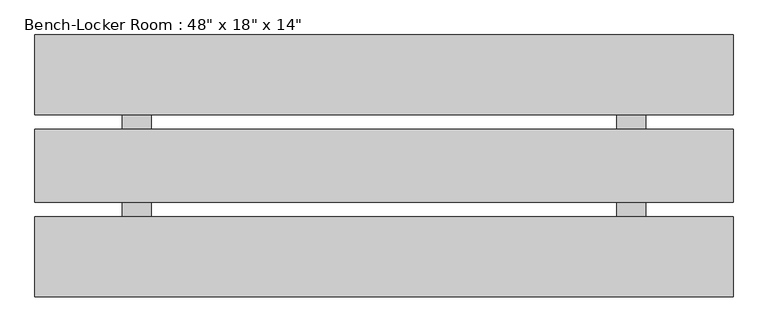
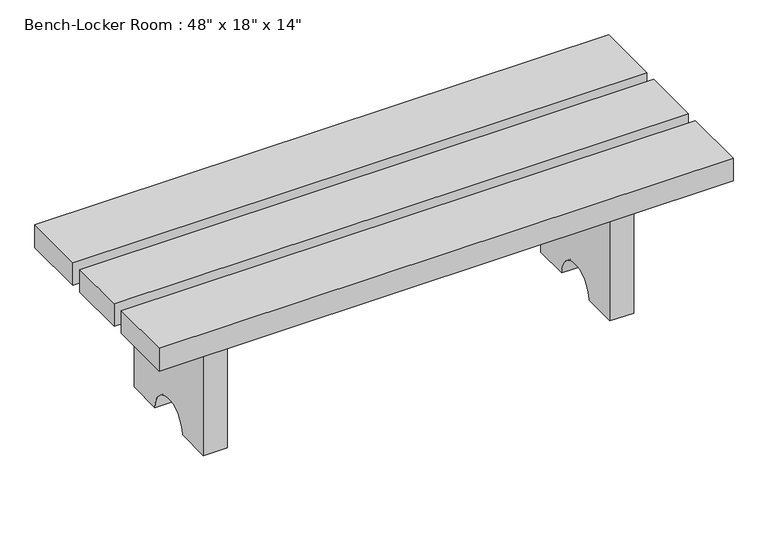
"""IFC4 building model written with IfcOpenShell, lengths in millimetres: furniture geometry."""

from ifc_helpers import new_model, si_unit, point, frame, frame_2d, origin, place, context, project, spatial, polyline, circle_curve, trimmed, segment, composite_curve, outline, extrude, source, transform, mapped, element, save


def furniture_39ce88ff(model_context):
    return source(origin(), model_context, "Body", "SweptSolid", [
        extrude(outline(composite_curve([segment(polyline([(-307.7147541, 0.0), (-307.7147541, 304.8), (-53.7147541, 304.8), (-53.7147541, 0.0), (-129.9147541, 0.0)]), True, "CONTINUOUS"), segment(trimmed(circle_curve(frame_2d((-180.7147541, 0.0)), 50.8), [point((-129.9147541, 0.0))], [point((-231.5147541, 0.0))], True, "CARTESIAN"), True, "CONTINUOUS"), segment(polyline([(-231.5147541, 0.0), (-307.7147541, 0.0)]), True, "CONTINUOUS")], self_intersect=False)), frame((251.0852459, 0.0, 0.0), z_axis=(1.0, 0.0, 0.0), x_axis=(0.0, 1.0, 0.0)), (0.0, 0.0, 1.0), 50.8),
        extrude(outline(composite_curve([segment(polyline([(-53.7147541, 0.0), (-129.9147541, 0.0)]), True, "CONTINUOUS"), segment(trimmed(circle_curve(frame_2d((-180.7147541, 0.0)), 50.8), [point((-129.9147541, 0.0))], [point((-231.5147541, 0.0))], True, "CARTESIAN"), True, "CONTINUOUS"), segment(polyline([(-231.5147541, 0.0), (-307.7147541, 0.0), (-307.7147541, 304.8), (-53.7147541, 304.8), (-53.7147541, 0.0)]), True, "CONTINUOUS")], self_intersect=False)), frame((-612.5147541, 0.0, 0.0), z_axis=(1.0, 0.0, 0.0), x_axis=(0.0, 1.0, 0.0)), (0.0, 0.0, 1.0), 50.8),
        extrude(outline(polyline([(454.2852459, 47.8852459), (454.2852459, -91.8147541), (-764.9147541, -91.8147541), (-764.9147541, 47.8852459), (454.2852459, 47.8852459)])), frame((0.0, 0.0, 304.8), z_axis=(0.0, 0.0, 1.0), x_axis=(1.0, 0.0, 0.0)), (0.0, 0.0, 1.0), 50.8),
        extrude(outline(polyline([(454.2852459, -409.3147541), (-764.9147541, -409.3147541), (-764.9147541, -269.6147541), (454.2852459, -269.6147541), (454.2852459, -409.3147541)])), frame((0.0, 0.0, 304.8), z_axis=(0.0, 0.0, 1.0), x_axis=(1.0, 0.0, 0.0)), (0.0, 0.0, 1.0), 50.8),
        extrude(outline(polyline([(454.2852459, -117.2147541), (454.2852459, -244.2147541), (-764.9147541, -244.2147541), (-764.9147541, -117.2147541), (454.2852459, -117.2147541)])), frame((0.0, 0.0, 304.8), z_axis=(0.0, 0.0, 1.0), x_axis=(1.0, 0.0, 0.0)), (0.0, 0.0, 1.0), 50.8),
    ])


if __name__ == "__main__":
    model = new_model("IFC4")
    model_context = context("Model", 3, world=origin())
    ifc_project = project(units=[si_unit("LENGTHUNIT", "METRE", prefix="MILLI")], contexts=[model_context])
    site = spatial("IfcSite", under=ifc_project)
    building = spatial("IfcBuilding", under=site)
    placement = place(None, origin())
    furniture_shape = furniture_39ce88ff(model_context)
    element("IfcFurniture", 1, ObjectType="Bench-Locker Room : 48\" x 18\" x 14\"", at=placement, inside=building, context=model_context, shape_type="MappedRepresentation", body=[
        mapped(furniture_shape, transform((0.0, 0.0, 0.0), x_axis=(1.0, 0.0, 0.0), y_axis=(0.0, 1.0, 0.0), z_axis=(0.0, 0.0, 1.0))),
    ])
    save(model, "model.ifc")

# Revit data of these elements
# Type "Bench-Locker Room : 48\" x 18\" x 14\""
#   Assembly Code = "E2020200"
#   Depth = 1' - 6"
#   Height = 1' - 2"
#   Width = 4' - 0"
#   Bench Material = Cherry
#   Default Elevation = 0
# Element 1 (IfcFurniture, "Bench-Locker Room : 48\" x 18\" x 14\"")
#   Materials on its faces: "Cherry"
# Materials
#   "Cherry": class "Wood", colour RGB 226 177 128, transparency 0, Description = "Prunus Serotina", Cost = 0
